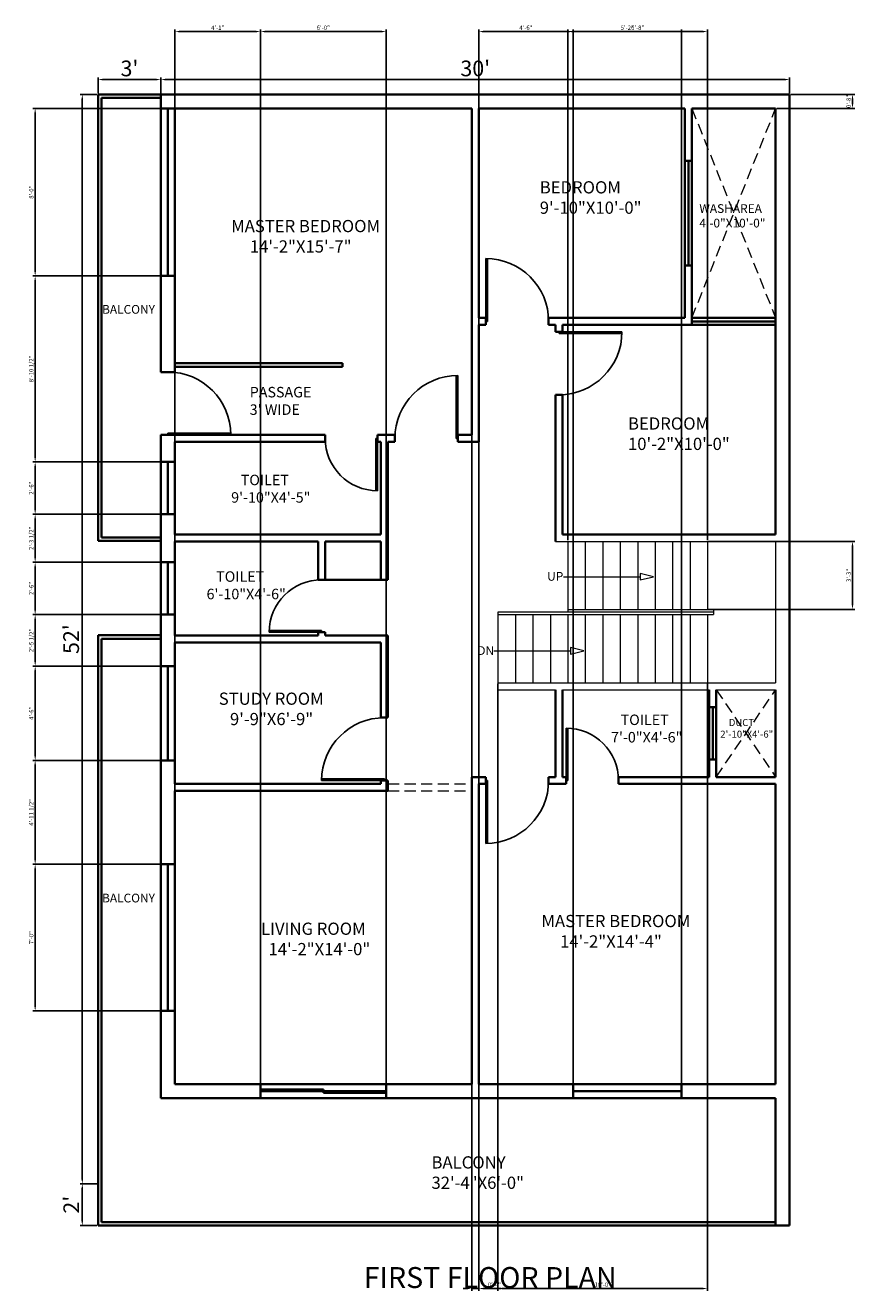
# Model space of a CAD drawing. Units: inches. Extents: x 1566 to 2546, y 1087 to 2705.
# Tile 27 of 27: x 2072 to 2546, y 1980 to 2705. Entities that reach past the tile are written whole.
import ezdxf

# ---------------------------------------------------------------- set-up
doc = ezdxf.new("R2010")
doc.units = ezdxf.units.IN
doc.linetypes.add('DASHED', pattern=[19.05, 12.7, -6.35])
for name, color, linetype, lineweight in [('A-ANNO-DIMS', 2, 'Continuous', 18), ('A-ANNO-TEXT', 7, 'Continuous', 18), ('A-AREA-IDEN', 7, 'Continuous', 18), ('A-DOOR', 4, 'Continuous', 25), ('A-FLOR-OVHD', 8, 'DASHED', 18), ('A-FLOR-STRS', 3, 'Continuous', 18), ('A-WALL', 7, 'Continuous', 35)]:
    doc.layers.add(name, color=color, linetype=linetype, lineweight=lineweight)
doc.styles.get("Standard").update_dxf_attribs({"font": 'arial.ttf'})
doc.dimstyles.new('ISO-25', dxfattribs={"dimtxt": 2.5, "dimasz": 2.5, "dimexe": 1.25, "dimexo": 0.625, "dimtad": 1, "dimtxsty": 'Standard', "dimcen": 2.5, "dimadec": 0, "dimazin": 0, "dimtfac": 1, "dimtmove": 0, "dimatfit": 3, "dimfxl": 1, "dimarcsym": 0})

# ---------------------------------------------------------------- blocks, each defined once
blk = doc.blocks.new('*D17')
at = {"layer": 'A-ANNO-DIMS', "color": 0, "lineweight": -2, "transparency": 16777216}
for p, q in [((2113.17, 2665.97), (2113.17, 2675.12)), ((2149.17, 2665.97), (2149.17, 2675.12)), ((2115.67, 2673.87), (2146.67, 2673.87))]:
    blk.add_line(p, q, dxfattribs=at)
at = {"layer": 'A-ANNO-DIMS', "color": 0, "transparency": 16777216}
for points in [[(2115.67, 2674.28), (2115.67, 2673.45), (2113.17, 2673.87)], [(2146.67, 2674.28), (2146.67, 2673.45), (2149.17, 2673.87)]]:
    blk.add_solid(points, dxfattribs=at)
at = {"layer": 'Defpoints', "color": 0, "transparency": 16777216}
for p in [(2149.17, 2673.87), (2113.17, 2665.35), (2149.17, 2665.35)]:
    blk.add_point(p, dxfattribs=at)
at = {"layer": 'A-ANNO-DIMS', "color": 0, "transparency": 16777216, "insert": (2131.17, 2679.09), "char_height": 9, "attachment_point": 5}
blk.add_mtext("3'", dxfattribs=at)
blk = doc.blocks.new('*D18')
at = {"layer": 'A-ANNO-DIMS', "color": 0, "lineweight": -2, "transparency": 16777216}
for p, q in [((2149.17, 2665.97), (2149.17, 2675.12)), ((2509.17, 2665.97), (2509.17, 2675.12)), ((2151.67, 2673.87), (2506.67, 2673.87))]:
    blk.add_line(p, q, dxfattribs=at)
at = {"layer": 'A-ANNO-DIMS', "color": 0, "transparency": 16777216}
for points in [[(2151.67, 2674.28), (2151.67, 2673.45), (2149.17, 2673.87)], [(2506.67, 2674.28), (2506.67, 2673.45), (2509.17, 2673.87)]]:
    blk.add_solid(points, dxfattribs=at)
at = {"layer": 'Defpoints', "color": 0, "transparency": 16777216}
for p in [(2509.17, 2673.87), (2149.17, 2665.35), (2509.17, 2665.35)]:
    blk.add_point(p, dxfattribs=at)
at = {"layer": 'A-ANNO-DIMS', "color": 0, "transparency": 16777216, "insert": (2329.17, 2679.09), "char_height": 9, "attachment_point": 5}
blk.add_mtext("30'", dxfattribs=at)
blk = doc.blocks.new('*D16')
at = {"layer": 'A-ANNO-DIMS', "color": 0, "lineweight": -2, "transparency": 16777216}
for p, q in [((2112.55, 2665.35), (2102.9, 2665.35)), ((2104.15, 2662.85), (2104.15, 2043.85)), ((2112.55, 2041.35), (2102.9, 2041.35))]:
    blk.add_line(p, q, dxfattribs=at)
at = {"layer": 'A-ANNO-DIMS', "color": 0, "transparency": 16777216}
for points in [[(2103.73, 2662.85), (2104.57, 2662.85), (2104.15, 2665.35)], [(2103.73, 2043.85), (2104.57, 2043.85), (2104.15, 2041.35)]]:
    blk.add_solid(points, dxfattribs=at)
at = {"layer": 'Defpoints', "color": 0, "transparency": 16777216}
for p in [(2113.17, 2665.35), (2104.15, 2041.35), (2113.17, 2041.35)]:
    blk.add_point(p, dxfattribs=at)
at = {"layer": 'A-ANNO-DIMS', "color": 0, "transparency": 16777216, "insert": (2098.93, 2353.35), "char_height": 9, "attachment_point": 5, "rotation": 90}
blk.add_mtext("52'", dxfattribs=at)
blk = doc.blocks.new('*D19')
at = {"layer": 'A-ANNO-DIMS', "color": 0, "lineweight": -2, "transparency": 16777216}
for p, q in [((2112.55, 2041.35), (2102.9, 2041.35)), ((2104.15, 2038.85), (2104.15, 2019.85)), ((2112.55, 2017.35), (2102.9, 2017.35))]:
    blk.add_line(p, q, dxfattribs=at)
at = {"layer": 'A-ANNO-DIMS', "color": 0, "transparency": 16777216}
for points in [[(2103.73, 2038.85), (2104.57, 2038.85), (2104.15, 2041.35)], [(2103.73, 2019.85), (2104.57, 2019.85), (2104.15, 2017.35)]]:
    blk.add_solid(points, dxfattribs=at)
at = {"layer": 'Defpoints', "color": 0, "transparency": 16777216}
for p in [(2113.17, 2041.35), (2104.15, 2017.35), (2113.17, 2017.35)]:
    blk.add_point(p, dxfattribs=at)
at = {"layer": 'A-ANNO-DIMS', "color": 0, "transparency": 16777216, "insert": (2099.01, 2029.35), "char_height": 9, "attachment_point": 5, "rotation": 90}
blk.add_mtext("2'", dxfattribs=at)
blk = doc.blocks.new('d1')
for p, q in [((3297.32, 1596.93), (3297.32, 1632.93)), ((3298.32, 1596.93), (3298.32, 1632.93)), ((3297.32, 1596.93), (3298.32, 1596.93))]:
    blk.add_line(p, q)
at = {"ltscale": 0.3}
blk.add_arc((3297.32, 1596.93), 36, 0, 90, dxfattribs=at)
blk = doc.blocks.new('d2')
for p, q in [((3364.08, 1632.29), (3364.08, 1602.29)), ((3365.08, 1632.29), (3365.08, 1602.29)), ((3364.08, 1602.29), (3365.08, 1602.29))]:
    blk.add_line(p, q)
at = {"ltscale": 0.3}
blk.add_arc((3364.08, 1602.29), 30, 0, 90, dxfattribs=at)
blk = doc.blocks.new('*D89')
at = {"layer": 'A-ANNO-DIMS', "color": 0, "lineweight": -2, "transparency": 16777216}
for p, q in [((2509.8, 2665.35), (2546.42, 2665.35)), ((2545.17, 2662.85), (2545.17, 2659.85)), ((2501.8, 2657.35), (2546.42, 2657.35))]:
    blk.add_line(p, q, dxfattribs=at)
at = {"layer": 'A-ANNO-DIMS', "color": 0, "transparency": 16777216}
for points in [[(2544.75, 2662.85), (2545.59, 2662.85), (2545.17, 2665.35)], [(2544.75, 2659.85), (2545.59, 2659.85), (2545.17, 2657.35)]]:
    blk.add_solid(points, dxfattribs=at)
at = {"layer": 'Defpoints', "color": 0, "transparency": 16777216}
for p in [(2509.17, 2665.35), (2501.17, 2657.35), (2545.17, 2657.35)]:
    blk.add_point(p, dxfattribs=at)
at = {"layer": 'A-ANNO-DIMS', "color": 0, "transparency": 16777216, "insert": (2543.27, 2661.35), "char_height": 2.5, "attachment_point": 5, "rotation": 90}
blk.add_mtext('0\'-8"', dxfattribs=at)
blk = doc.blocks.new('*D90')
at = {"layer": 'A-ANNO-DIMS', "color": 0, "lineweight": -2, "transparency": 16777216}
for p, q in [((2327.17, 2656.72), (2327.17, 1980.1)), ((2331.17, 2656.72), (2331.17, 1980.1)), ((2324.67, 1981.35), (2322.17, 1981.35)), ((2327.17, 1981.35), (2331.17, 1981.35)), ((2333.67, 1981.35), (2344.07, 1981.35))]:
    blk.add_line(p, q, dxfattribs=at)
at = {"layer": 'A-ANNO-DIMS', "color": 0, "transparency": 16777216}
for points in [[(2324.67, 1981.76), (2324.67, 1980.93), (2327.17, 1981.35)], [(2333.67, 1981.76), (2333.67, 1980.93), (2331.17, 1981.35)]]:
    blk.add_solid(points, dxfattribs=at)
at = {"layer": 'Defpoints', "color": 0, "transparency": 16777216}
for p in [(2327.17, 2657.35), (2331.17, 2657.35), (2331.17, 1981.35)]:
    blk.add_point(p, dxfattribs=at)
at = {"layer": 'A-ANNO-DIMS', "color": 0, "transparency": 16777216, "insert": (2340.12, 1983.25), "char_height": 2.5, "attachment_point": 5}
blk.add_mtext('0\'-4"', dxfattribs=at)
blk = doc.blocks.new('*D93')
at = {"layer": 'A-ANNO-DIMS', "color": 0, "lineweight": -2, "transparency": 16777216}
for p, q in [((2148.55, 2657.35), (2075.92, 2657.35)), ((2077.17, 2654.85), (2077.17, 2563.85)), ((2148.55, 2561.35), (2075.92, 2561.35))]:
    blk.add_line(p, q, dxfattribs=at)
at = {"layer": 'A-ANNO-DIMS', "color": 0, "transparency": 16777216}
for points in [[(2076.75, 2654.85), (2077.59, 2654.85), (2077.17, 2657.35)], [(2076.75, 2563.85), (2077.59, 2563.85), (2077.17, 2561.35)]]:
    blk.add_solid(points, dxfattribs=at)
at = {"layer": 'Defpoints', "color": 0, "transparency": 16777216}
for p in [(2149.17, 2657.35), (2077.17, 2561.35), (2149.17, 2561.35)]:
    blk.add_point(p, dxfattribs=at)
at = {"layer": 'A-ANNO-DIMS', "color": 0, "transparency": 16777216, "insert": (2075.27, 2609.35), "char_height": 2.5, "attachment_point": 5, "rotation": 90}
blk.add_mtext('8\'-0"', dxfattribs=at)
blk = doc.blocks.new('*D94')
at = {"layer": 'A-ANNO-DIMS', "color": 0, "lineweight": -2, "transparency": 16777216}
for p, q in [((2148.55, 2561.35), (2075.92, 2561.35)), ((2077.17, 2558.85), (2077.17, 2457.35)), ((2148.55, 2454.85), (2075.92, 2454.85))]:
    blk.add_line(p, q, dxfattribs=at)
at = {"layer": 'A-ANNO-DIMS', "color": 0, "transparency": 16777216}
for points in [[(2076.75, 2558.85), (2077.59, 2558.85), (2077.17, 2561.35)], [(2076.75, 2457.35), (2077.59, 2457.35), (2077.17, 2454.85)]]:
    blk.add_solid(points, dxfattribs=at)
at = {"layer": 'Defpoints', "color": 0, "transparency": 16777216}
for p in [(2149.17, 2561.35), (2077.17, 2454.85), (2149.17, 2454.85)]:
    blk.add_point(p, dxfattribs=at)
at = {"layer": 'A-ANNO-DIMS', "color": 0, "transparency": 16777216, "insert": (2075.25, 2508.1), "char_height": 2.5, "attachment_point": 5, "rotation": 90}
blk.add_mtext('8\'-10 1/2"', dxfattribs=at)
blk = doc.blocks.new('*D95')
at = {"layer": 'A-ANNO-DIMS', "color": 0, "lineweight": -2, "transparency": 16777216}
for p, q in [((2148.55, 2454.85), (2075.92, 2454.85)), ((2077.17, 2452.35), (2077.17, 2427.35)), ((2148.55, 2424.85), (2075.92, 2424.85))]:
    blk.add_line(p, q, dxfattribs=at)
at = {"layer": 'A-ANNO-DIMS', "color": 0, "transparency": 16777216}
for points in [[(2076.75, 2452.35), (2077.59, 2452.35), (2077.17, 2454.85)], [(2076.75, 2427.35), (2077.59, 2427.35), (2077.17, 2424.85)]]:
    blk.add_solid(points, dxfattribs=at)
at = {"layer": 'Defpoints', "color": 0, "transparency": 16777216}
for p in [(2149.17, 2454.85), (2077.17, 2424.85), (2149.17, 2424.85)]:
    blk.add_point(p, dxfattribs=at)
at = {"layer": 'A-ANNO-DIMS', "color": 0, "transparency": 16777216, "insert": (2075.27, 2439.85), "char_height": 2.5, "attachment_point": 5, "rotation": 90}
blk.add_mtext('2\'-6"', dxfattribs=at)
blk = doc.blocks.new('*D96')
at = {"layer": 'A-ANNO-DIMS', "color": 0, "lineweight": -2, "transparency": 16777216}
for p, q in [((2148.55, 2424.85), (2075.92, 2424.85)), ((2077.17, 2422.35), (2077.17, 2399.85)), ((2148.55, 2397.35), (2075.92, 2397.35))]:
    blk.add_line(p, q, dxfattribs=at)
at = {"layer": 'A-ANNO-DIMS', "color": 0, "transparency": 16777216}
for points in [[(2076.75, 2422.35), (2077.59, 2422.35), (2077.17, 2424.85)], [(2076.75, 2399.85), (2077.59, 2399.85), (2077.17, 2397.35)]]:
    blk.add_solid(points, dxfattribs=at)
at = {"layer": 'Defpoints', "color": 0, "transparency": 16777216}
for p in [(2149.17, 2424.85), (2077.17, 2397.35), (2149.17, 2397.35)]:
    blk.add_point(p, dxfattribs=at)
at = {"layer": 'A-ANNO-DIMS', "color": 0, "transparency": 16777216, "insert": (2075.25, 2411.1), "char_height": 2.5, "attachment_point": 5, "rotation": 90}
blk.add_mtext('2\'-3 1/2"', dxfattribs=at)
blk = doc.blocks.new('*D97')
at = {"layer": 'A-ANNO-DIMS', "color": 0, "lineweight": -2, "transparency": 16777216}
for p, q in [((2148.55, 2397.35), (2075.92, 2397.35)), ((2077.17, 2394.85), (2077.17, 2369.85)), ((2148.55, 2367.35), (2075.92, 2367.35))]:
    blk.add_line(p, q, dxfattribs=at)
at = {"layer": 'A-ANNO-DIMS', "color": 0, "transparency": 16777216}
for points in [[(2076.75, 2394.85), (2077.59, 2394.85), (2077.17, 2397.35)], [(2076.75, 2369.85), (2077.59, 2369.85), (2077.17, 2367.35)]]:
    blk.add_solid(points, dxfattribs=at)
at = {"layer": 'Defpoints', "color": 0, "transparency": 16777216}
for p in [(2149.17, 2397.35), (2077.17, 2367.35), (2149.17, 2367.35)]:
    blk.add_point(p, dxfattribs=at)
at = {"layer": 'A-ANNO-DIMS', "color": 0, "transparency": 16777216, "insert": (2075.27, 2382.35), "char_height": 2.5, "attachment_point": 5, "rotation": 90}
blk.add_mtext('2\'-6"', dxfattribs=at)
blk = doc.blocks.new('*D98')
at = {"layer": 'A-ANNO-DIMS', "color": 0, "lineweight": -2, "transparency": 16777216}
for p, q in [((2148.55, 2367.35), (2075.92, 2367.35)), ((2077.17, 2364.85), (2077.17, 2340.35)), ((2148.55, 2337.85), (2075.92, 2337.85))]:
    blk.add_line(p, q, dxfattribs=at)
at = {"layer": 'A-ANNO-DIMS', "color": 0, "transparency": 16777216}
for points in [[(2076.75, 2364.85), (2077.59, 2364.85), (2077.17, 2367.35)], [(2076.75, 2340.35), (2077.59, 2340.35), (2077.17, 2337.85)]]:
    blk.add_solid(points, dxfattribs=at)
at = {"layer": 'Defpoints', "color": 0, "transparency": 16777216}
for p in [(2149.17, 2367.35), (2077.17, 2337.85), (2149.17, 2337.85)]:
    blk.add_point(p, dxfattribs=at)
at = {"layer": 'A-ANNO-DIMS', "color": 0, "transparency": 16777216, "insert": (2075.25, 2352.6), "char_height": 2.5, "attachment_point": 5, "rotation": 90}
blk.add_mtext('2\'-5 1/2"', dxfattribs=at)
blk = doc.blocks.new('*D99')
at = {"layer": 'A-ANNO-DIMS', "color": 0, "lineweight": -2, "transparency": 16777216}
for p, q in [((2148.55, 2337.85), (2075.92, 2337.85)), ((2077.17, 2335.35), (2077.17, 2286.35)), ((2148.55, 2283.85), (2075.92, 2283.85))]:
    blk.add_line(p, q, dxfattribs=at)
at = {"layer": 'A-ANNO-DIMS', "color": 0, "transparency": 16777216}
for points in [[(2076.75, 2335.35), (2077.59, 2335.35), (2077.17, 2337.85)], [(2076.75, 2286.35), (2077.59, 2286.35), (2077.17, 2283.85)]]:
    blk.add_solid(points, dxfattribs=at)
at = {"layer": 'Defpoints', "color": 0, "transparency": 16777216}
for p in [(2149.17, 2337.85), (2077.17, 2283.85), (2149.17, 2283.85)]:
    blk.add_point(p, dxfattribs=at)
at = {"layer": 'A-ANNO-DIMS', "color": 0, "transparency": 16777216, "insert": (2075.27, 2310.85), "char_height": 2.5, "attachment_point": 5, "rotation": 90}
blk.add_mtext('4\'-6"', dxfattribs=at)
blk = doc.blocks.new('*D100')
at = {"layer": 'A-ANNO-DIMS', "color": 0, "lineweight": -2, "transparency": 16777216}
for p, q in [((2148.55, 2283.85), (2075.92, 2283.85)), ((2077.17, 2281.35), (2077.17, 2226.85)), ((2148.55, 2224.35), (2075.92, 2224.35))]:
    blk.add_line(p, q, dxfattribs=at)
at = {"layer": 'A-ANNO-DIMS', "color": 0, "transparency": 16777216}
for points in [[(2076.75, 2281.35), (2077.59, 2281.35), (2077.17, 2283.85)], [(2076.75, 2226.85), (2077.59, 2226.85), (2077.17, 2224.35)]]:
    blk.add_solid(points, dxfattribs=at)
at = {"layer": 'Defpoints', "color": 0, "transparency": 16777216}
for p in [(2149.17, 2283.85), (2077.17, 2224.35), (2149.17, 2224.35)]:
    blk.add_point(p, dxfattribs=at)
at = {"layer": 'A-ANNO-DIMS', "color": 0, "transparency": 16777216, "insert": (2075.25, 2254.1), "char_height": 2.5, "attachment_point": 5, "rotation": 90}
blk.add_mtext('4\'-11 1/2"', dxfattribs=at)
blk = doc.blocks.new('*D101')
at = {"layer": 'A-ANNO-DIMS', "color": 0, "lineweight": -2, "transparency": 16777216}
for p, q in [((2148.55, 2224.35), (2075.92, 2224.35)), ((2077.17, 2221.85), (2077.17, 2142.85)), ((2148.55, 2140.35), (2075.92, 2140.35))]:
    blk.add_line(p, q, dxfattribs=at)
at = {"layer": 'A-ANNO-DIMS', "color": 0, "transparency": 16777216}
for points in [[(2076.75, 2221.85), (2077.59, 2221.85), (2077.17, 2224.35)], [(2076.75, 2142.85), (2077.59, 2142.85), (2077.17, 2140.35)]]:
    blk.add_solid(points, dxfattribs=at)
at = {"layer": 'Defpoints', "color": 0, "transparency": 16777216}
for p in [(2149.17, 2224.35), (2077.17, 2140.35), (2149.17, 2140.35)]:
    blk.add_point(p, dxfattribs=at)
at = {"layer": 'A-ANNO-DIMS', "color": 0, "transparency": 16777216, "insert": (2075.27, 2182.35), "char_height": 2.5, "attachment_point": 5, "rotation": 90}
blk.add_mtext('7\'-0"', dxfattribs=at)
blk = doc.blocks.new('*D102')
at = {"layer": 'A-ANNO-DIMS', "color": 0, "lineweight": -2, "transparency": 16777216}
for p, q in [((2157.17, 2098.97), (2157.17, 2702.6)), ((2159.67, 2701.35), (2203.67, 2701.35)), ((2206.17, 2098.97), (2206.17, 2702.6))]:
    blk.add_line(p, q, dxfattribs=at)
at = {"layer": 'A-ANNO-DIMS', "color": 0, "transparency": 16777216}
for points in [[(2159.67, 2701.76), (2159.67, 2700.93), (2157.17, 2701.35)], [(2203.67, 2701.76), (2203.67, 2700.93), (2206.17, 2701.35)]]:
    blk.add_solid(points, dxfattribs=at)
at = {"layer": 'Defpoints', "color": 0, "transparency": 16777216}
for p in [(2206.17, 2701.35), (2157.17, 2098.35), (2206.17, 2098.35)]:
    blk.add_point(p, dxfattribs=at)
at = {"layer": 'A-ANNO-DIMS', "color": 0, "transparency": 16777216, "insert": (2181.67, 2703.23), "char_height": 2.5, "attachment_point": 5}
blk.add_mtext('4\'-1"', dxfattribs=at)
blk = doc.blocks.new('*D103')
at = {"layer": 'A-ANNO-DIMS', "color": 0, "lineweight": -2, "transparency": 16777216}
for p, q in [((2206.17, 2098.97), (2206.17, 2702.6)), ((2208.67, 2701.35), (2275.67, 2701.35)), ((2278.17, 2098.97), (2278.17, 2702.6))]:
    blk.add_line(p, q, dxfattribs=at)
at = {"layer": 'A-ANNO-DIMS', "color": 0, "transparency": 16777216}
for points in [[(2208.67, 2701.76), (2208.67, 2700.93), (2206.17, 2701.35)], [(2275.67, 2701.76), (2275.67, 2700.93), (2278.17, 2701.35)]]:
    blk.add_solid(points, dxfattribs=at)
at = {"layer": 'Defpoints', "color": 0, "transparency": 16777216}
for p in [(2278.17, 2701.35), (2206.17, 2098.35), (2278.17, 2098.35)]:
    blk.add_point(p, dxfattribs=at)
at = {"layer": 'A-ANNO-DIMS', "color": 0, "transparency": 16777216, "insert": (2242.17, 2703.25), "char_height": 2.5, "attachment_point": 5}
blk.add_mtext('6\'-0"', dxfattribs=at)
blk = doc.blocks.new('*D104')
at = {"layer": 'A-ANNO-DIMS', "color": 0, "lineweight": -2, "transparency": 16777216}
for p, q in [((2331.17, 2098.97), (2331.17, 2702.6)), ((2333.67, 2701.35), (2382.67, 2701.35)), ((2385.17, 2098.97), (2385.17, 2702.6))]:
    blk.add_line(p, q, dxfattribs=at)
at = {"layer": 'A-ANNO-DIMS', "color": 0, "transparency": 16777216}
for points in [[(2333.67, 2701.76), (2333.67, 2700.93), (2331.17, 2701.35)], [(2382.67, 2701.76), (2382.67, 2700.93), (2385.17, 2701.35)]]:
    blk.add_solid(points, dxfattribs=at)
at = {"layer": 'Defpoints', "color": 0, "transparency": 16777216}
for p in [(2385.17, 2701.35), (2331.17, 2098.35), (2385.17, 2098.35)]:
    blk.add_point(p, dxfattribs=at)
at = {"layer": 'A-ANNO-DIMS', "color": 0, "transparency": 16777216, "insert": (2358.17, 2703.25), "char_height": 2.5, "attachment_point": 5}
blk.add_mtext('4\'-6"', dxfattribs=at)
blk = doc.blocks.new('*D105')
at = {"layer": 'A-ANNO-DIMS', "color": 0, "lineweight": -2, "transparency": 16777216}
for p, q in [((2385.17, 2098.97), (2385.17, 2702.6)), ((2387.67, 2701.35), (2444.67, 2701.35)), ((2447.17, 2098.97), (2447.17, 2702.6))]:
    blk.add_line(p, q, dxfattribs=at)
at = {"layer": 'A-ANNO-DIMS', "color": 0, "transparency": 16777216}
for points in [[(2387.67, 2701.76), (2387.67, 2700.93), (2385.17, 2701.35)], [(2444.67, 2701.76), (2444.67, 2700.93), (2447.17, 2701.35)]]:
    blk.add_solid(points, dxfattribs=at)
at = {"layer": 'Defpoints', "color": 0, "transparency": 16777216}
for p in [(2447.17, 2701.35), (2385.17, 2098.35), (2447.17, 2098.35)]:
    blk.add_point(p, dxfattribs=at)
at = {"layer": 'A-ANNO-DIMS', "color": 0, "transparency": 16777216, "insert": (2416.17, 2703.25), "char_height": 2.5, "attachment_point": 5}
blk.add_mtext('5\'-2"', dxfattribs=at)
blk = doc.blocks.new('*D106')
at = {"layer": 'A-ANNO-DIMS', "color": 0, "lineweight": -2, "transparency": 16777216}
for p, q in [((2382.17, 2409.97), (2382.17, 2702.6)), ((2384.67, 2701.35), (2459.67, 2701.35)), ((2462.17, 2409.97), (2462.17, 2702.6))]:
    blk.add_line(p, q, dxfattribs=at)
at = {"layer": 'A-ANNO-DIMS', "color": 0, "transparency": 16777216}
for points in [[(2384.67, 2701.76), (2384.67, 2700.93), (2382.17, 2701.35)], [(2459.67, 2701.76), (2459.67, 2700.93), (2462.17, 2701.35)]]:
    blk.add_solid(points, dxfattribs=at)
at = {"layer": 'Defpoints', "color": 0, "transparency": 16777216}
for p in [(2462.17, 2701.35), (2382.17, 2409.35), (2462.17, 2409.35)]:
    blk.add_point(p, dxfattribs=at)
at = {"layer": 'A-ANNO-DIMS', "color": 0, "transparency": 16777216, "insert": (2422.17, 2703.25), "char_height": 2.5, "attachment_point": 5}
blk.add_mtext('6\'-8"', dxfattribs=at)
blk = doc.blocks.new('*D107')
at = {"layer": 'A-ANNO-DIMS', "color": 0, "lineweight": -2, "transparency": 16777216}
for p, q in [((2462.8, 2409.35), (2546.42, 2409.35)), ((2545.17, 2406.85), (2545.17, 2372.85)), ((2462.8, 2370.35), (2546.42, 2370.35))]:
    blk.add_line(p, q, dxfattribs=at)
at = {"layer": 'A-ANNO-DIMS', "color": 0, "transparency": 16777216}
for points in [[(2544.75, 2406.85), (2545.59, 2406.85), (2545.17, 2409.35)], [(2544.75, 2372.85), (2545.59, 2372.85), (2545.17, 2370.35)]]:
    blk.add_solid(points, dxfattribs=at)
at = {"layer": 'Defpoints', "color": 0, "transparency": 16777216}
for p in [(2462.17, 2409.35), (2462.17, 2370.35), (2545.17, 2370.35)]:
    blk.add_point(p, dxfattribs=at)
at = {"layer": 'A-ANNO-DIMS', "color": 0, "transparency": 16777216, "insert": (2543.27, 2389.85), "char_height": 2.5, "attachment_point": 5, "rotation": 90}
blk.add_mtext('3\'-3"', dxfattribs=at)
blk = doc.blocks.new('*D108')
at = {"layer": 'A-ANNO-DIMS', "color": 0, "lineweight": -2, "transparency": 16777216}
for p, q in [((2342.17, 2327.72), (2342.17, 1980.1)), ((2462.17, 2327.72), (2462.17, 1980.1)), ((2344.67, 1981.35), (2459.67, 1981.35))]:
    blk.add_line(p, q, dxfattribs=at)
at = {"layer": 'A-ANNO-DIMS', "color": 0, "transparency": 16777216}
for points in [[(2344.67, 1981.76), (2344.67, 1980.93), (2342.17, 1981.35)], [(2459.67, 1981.76), (2459.67, 1980.93), (2462.17, 1981.35)]]:
    blk.add_solid(points, dxfattribs=at)
at = {"layer": 'Defpoints', "color": 0, "transparency": 16777216}
for p in [(2342.17, 2328.35), (2462.17, 2328.35), (2462.17, 1981.35)]:
    blk.add_point(p, dxfattribs=at)
at = {"layer": 'A-ANNO-DIMS', "color": 0, "transparency": 16777216, "insert": (2402.17, 1983.25), "char_height": 2.5, "attachment_point": 5}
blk.add_mtext('10\'-0"', dxfattribs=at)

msp = doc.modelspace()

# ---------------------------------------------------------------- linework, layer by layer
at = {"layer": 'A-FLOR-OVHD', "ltscale": 0.5}
for p, q in [((2453.17, 2657.35), (2501.17, 2537.35)), ((2453.17, 2537.35), (2501.17, 2657.35)), ((2467.17, 2324.35), (2501.17, 2274.35)), ((2467.17, 2274.35), (2501.17, 2324.35)), ((2279.17, 2270.35), (2327.17, 2270.35)), ((2279.17, 2266.35), (2327.17, 2266.35))]:
    msp.add_line(p, q, dxfattribs=at)
at = {"layer": 'A-FLOR-STRS'}
for p, q in [((2375.17, 2409.35), (2501.17, 2409.35)), ((2382.17, 2409.35), (2382.17, 2368.85)), ((2392.17, 2409.35), (2392.17, 2370.35)), ((2402.17, 2409.35), (2402.17, 2370.35)), ((2412.17, 2409.35), (2412.17, 2370.35)), ((2422.17, 2409.35), (2422.17, 2370.35)), ((2432.17, 2409.35), (2432.17, 2370.35)), ((2442.17, 2409.35), (2442.17, 2370.35)), ((2452.17, 2409.35), (2452.17, 2370.35)), ((2462.17, 2409.35), (2462.17, 2370.35)), ((2501.17, 2409.35), (2501.17, 2328.35)), ((2379.74, 2389.1), (2423.62, 2389.1)), ((2382.17, 2370.35), (2465.67, 2370.35)), ((2465.67, 2370.35), (2465.67, 2367.35)), ((2342.17, 2368.85), (2342.17, 2324.35)), ((2465.67, 2368.85), (2342.17, 2368.85)), ((2342.17, 2367.35), (2465.67, 2367.35)), ((2352.17, 2367.35), (2352.17, 2328.35)), ((2362.17, 2367.35), (2362.17, 2328.35)), ((2372.17, 2367.35), (2372.17, 2328.35)), ((2382.17, 2367.35), (2382.17, 2366.85)), ((2382.17, 2367.35), (2382.17, 2328.35)), ((2392.17, 2367.35), (2392.17, 2328.35)), ((2402.17, 2367.35), (2402.17, 2328.35)), ((2412.17, 2367.35), (2412.17, 2328.35)), ((2422.17, 2367.35), (2422.17, 2328.35)), ((2432.17, 2367.35), (2432.17, 2328.35)), ((2442.17, 2367.35), (2442.17, 2328.35)), ((2452.17, 2367.35), (2452.17, 2328.35)), ((2462.17, 2367.35), (2462.17, 2328.35)), ((2339.74, 2346.6), (2383.62, 2346.6)), ((2342.17, 2328.35), (2501.17, 2328.35)), ((2342.17, 2324.35), (2375.17, 2324.35)), ((2379.17, 2324.35), (2463.17, 2324.35)), ((2467.17, 2324.35), (2501.17, 2324.35))]:
    msp.add_line(p, q, dxfattribs=at)
for points in [[(2431.27, 2389.1), (2423.62, 2390.95), (2423.62, 2387.24)], [(2391.27, 2346.6), (2383.62, 2348.45), (2383.62, 2344.74)]]:
    msp.add_lwpolyline(points, close=True, dxfattribs=at)
at = {"layer": 'A-WALL'}
for p, q in [((2113.17, 2409.59), (2113.17, 2665.35)), ((2113.17, 2665.35), (2149.17, 2665.35)), ((2115.17, 2411.59), (2115.17, 2663.35)), ((2115.17, 2663.35), (2149.17, 2663.35)), ((2149.17, 2506.35), (2149.17, 2665.35)), ((2149.17, 2665.35), (2509.17, 2665.35)), ((2509.17, 2665.35), (2509.17, 2017.35)), ((2149.17, 2657.35), (2327.17, 2657.35)), ((2153.17, 2561.35), (2153.17, 2657.35)), ((2157.17, 2506.35), (2157.17, 2657.35)), ((2327.17, 2470.35), (2327.17, 2657.35)), ((2331.17, 2657.35), (2449.17, 2657.35)), ((2331.17, 2537.35), (2331.17, 2657.35)), ((2449.17, 2537.35), (2449.17, 2657.35)), ((2453.17, 2657.35), (2501.17, 2657.35)), ((2453.17, 2533.35), (2453.17, 2657.35)), ((2501.17, 2657.35), (2501.17, 2413.35)), ((2449.17, 2627.35), (2453.17, 2627.35)), ((2451.17, 2627.35), (2451.17, 2567.35)), ((2449.17, 2567.35), (2453.17, 2567.35)), ((2149.17, 2561.35), (2157.17, 2561.35)), ((2331.17, 2537.35), (2335.17, 2537.35)), ((2335.17, 2533.35), (2335.17, 2537.35)), ((2371.17, 2537.35), (2449.17, 2537.35)), ((2371.17, 2533.35), (2371.17, 2537.35)), ((2453.17, 2537.35), (2501.17, 2537.35)), ((2331.17, 2533.35), (2335.17, 2533.35)), ((2331.17, 2466.35), (2331.17, 2533.35)), ((2371.17, 2533.35), (2375.17, 2533.35)), ((2375.17, 2533.35), (2375.17, 2529.35)), ((2379.17, 2533.35), (2501.17, 2533.35)), ((2379.17, 2533.35), (2379.17, 2529.35)), ((2501.17, 2535.35), (2453.17, 2535.35)), ((2375.17, 2529.35), (2379.17, 2529.35)), ((2157.17, 2511.35), (2253.17, 2511.35)), ((2157.17, 2509.35), (2253.17, 2509.35)), ((2253.17, 2509.35), (2253.17, 2511.35)), ((2149.17, 2506.35), (2157.17, 2506.35)), ((2375.17, 2493.35), (2379.17, 2493.35)), ((2375.17, 2493.35), (2375.17, 2409.35)), ((2379.17, 2493.35), (2379.17, 2413.35)), ((2149.17, 2090.35), (2149.17, 2470.35)), ((2149.17, 2470.35), (2243.17, 2470.35)), ((2157.17, 2466.35), (2243.17, 2466.35)), ((2157.17, 2413.35), (2157.17, 2466.35)), ((2243.17, 2466.35), (2243.17, 2470.35)), ((2273.17, 2470.35), (2275.17, 2470.35)), ((2273.17, 2466.35), (2273.17, 2470.35)), ((2273.17, 2466.35), (2275.17, 2466.35)), ((2275.17, 2470.35), (2283.17, 2470.35)), ((2275.17, 2413.35), (2275.17, 2466.35)), ((2279.17, 2466.35), (2283.17, 2466.35)), ((2279.17, 2387.35), (2279.17, 2466.35)), ((2283.17, 2466.35), (2283.17, 2470.35)), ((2319.17, 2470.35), (2327.17, 2470.35)), ((2319.17, 2466.35), (2319.17, 2470.35)), ((2319.17, 2466.35), (2331.17, 2466.35)), ((2157.17, 2454.85), (2149.17, 2454.85)), ((2153.17, 2454.85), (2153.17, 2424.85)), ((2157.17, 2424.85), (2149.17, 2424.85)), ((2149.17, 2409.59), (2113.17, 2409.59)), ((2149.17, 2411.59), (2115.17, 2411.59)), ((2157.17, 2413.35), (2275.17, 2413.35)), ((2157.17, 2409.35), (2239.17, 2409.35)), ((2157.17, 2355.35), (2157.17, 2409.35)), ((2239.17, 2387.35), (2239.17, 2409.35)), ((2243.17, 2409.35), (2275.17, 2409.35)), ((2243.17, 2387.35), (2243.17, 2409.35)), ((2275.17, 2387.35), (2275.17, 2409.35)), ((2379.17, 2413.35), (2501.17, 2413.35)), ((2157.17, 2397.35), (2149.17, 2397.35)), ((2153.17, 2397.35), (2153.17, 2367.35)), ((2239.17, 2387.35), (2279.17, 2387.35)), ((2157.17, 2367.35), (2149.17, 2367.35)), ((2239.17, 2355.35), (2239.17, 2357.35)), ((2239.17, 2357.35), (2243.17, 2357.35)), ((2243.17, 2355.35), (2243.17, 2357.35)), ((2149.17, 2355.56), (2113.17, 2355.56)), ((2113.17, 2355.56), (2113.17, 2017.35)), ((2149.17, 2353.56), (2115.17, 2353.56)), ((2115.17, 2353.56), (2115.17, 2019.35)), ((2157.17, 2355.35), (2239.17, 2355.35)), ((2157.17, 2351.35), (2275.17, 2351.35)), ((2157.17, 2270.35), (2157.17, 2351.35)), ((2243.17, 2355.35), (2279.17, 2355.35)), ((2275.17, 2308.35), (2275.17, 2351.35)), ((2279.17, 2308.35), (2279.17, 2355.35)), ((2157.17, 2337.85), (2149.17, 2337.85)), ((2153.17, 2337.85), (2153.17, 2283.85)), ((2375.17, 2324.35), (2375.17, 2274.35)), ((2379.17, 2324.35), (2379.17, 2274.35)), ((2463.17, 2324.35), (2463.17, 2274.35)), ((2467.17, 2324.35), (2467.17, 2274.35)), ((2501.17, 2324.35), (2501.17, 2274.35)), ((2463.17, 2314.35), (2467.17, 2314.35)), ((2465.17, 2314.35), (2465.17, 2284.35)), ((2275.17, 2308.35), (2279.17, 2308.35)), ((2157.17, 2283.85), (2149.17, 2283.85)), ((2463.17, 2284.35), (2467.17, 2284.35)), ((2157.17, 2270.35), (2275.17, 2270.35)), ((2275.17, 2272.35), (2279.17, 2272.35)), ((2275.17, 2270.35), (2275.17, 2272.35)), ((2279.17, 2266.35), (2279.17, 2272.35)), ((2327.17, 2274.35), (2335.17, 2274.35)), ((2327.17, 2098.35), (2327.17, 2274.35)), ((2331.17, 2270.35), (2335.17, 2270.35)), ((2331.17, 2098.35), (2331.17, 2270.35)), ((2335.17, 2270.35), (2335.17, 2274.35)), ((2371.17, 2274.35), (2375.17, 2274.35)), ((2371.17, 2270.35), (2371.17, 2274.35)), ((2371.17, 2270.35), (2381.17, 2270.35)), ((2379.17, 2274.35), (2381.17, 2274.35)), ((2381.17, 2274.35), (2381.17, 2270.35)), ((2411.17, 2274.35), (2463.17, 2274.35)), ((2411.17, 2274.35), (2411.17, 2270.35)), ((2411.17, 2270.35), (2501.17, 2270.35)), ((2467.17, 2274.35), (2501.17, 2274.35)), ((2501.17, 2270.35), (2501.17, 2098.35)), ((2157.17, 2266.35), (2279.17, 2266.35)), ((2157.17, 2098.35), (2157.17, 2266.35)), ((2157.17, 2224.35), (2149.17, 2224.35)), ((2153.17, 2224.35), (2153.17, 2140.35)), ((2157.17, 2140.35), (2149.17, 2140.35)), ((2157.17, 2098.35), (2327.17, 2098.35)), ((2206.17, 2098.35), (2206.17, 2090.35)), ((2206.17, 2095.35), (2242.17, 2095.35)), ((2242.17, 2095.35), (2242.17, 2093.35)), ((2278.17, 2098.35), (2278.17, 2090.35)), ((2331.17, 2098.35), (2501.17, 2098.35)), ((2385.17, 2098.35), (2385.17, 2090.35)), ((2447.17, 2098.35), (2447.17, 2090.35)), ((2149.17, 2090.35), (2501.17, 2090.35)), ((2206.17, 2094.35), (2278.17, 2094.35)), ((2242.17, 2093.35), (2278.17, 2093.35)), ((2385.17, 2094.35), (2447.17, 2094.35)), ((2501.17, 2090.35), (2501.17, 2017.35)), ((2113.17, 2017.35), (2509.17, 2017.35)), ((2115.17, 2019.35), (2501.17, 2019.35))]:
    msp.add_line(p, q, dxfattribs=at)

# ---------------------------------------------------------------- block references
at = {"layer": 'A-DOOR'}
for name, p in [('d1', (-962.15, 938.42)), ('d2', (-982.91, 670.05))]:
    msp.add_blockref(name, p, dxfattribs=at)
for name, p, rotation in [('d1', (780.25, 5826.67), 270), ('d2', (5637.25, 4070.64), 180), ('d2', (3843.46, -1006.73), 90), ('d1', (3874.1, -1024.98), 90)]:
    msp.add_blockref(name, p, dxfattribs=dict(at, rotation=rotation))
at = {"layer": 'A-DOOR', "xscale": -1}
for p, rotation in [((556.25, -826.98), 270), ((-962.15, 3869.27), 180)]:
    msp.add_blockref('d1', p, dxfattribs=dict(at, rotation=rotation))
msp.add_blockref('d1', (5616.49, 871.42), dxfattribs=at)

# ---------------------------------------------------------------- texts
at = {"layer": 'A-ANNO-TEXT'}
for s, p in [('UP', (2370.32, 2386.79)), ('DN', (2330.32, 2344.29))]:
    msp.add_text(s, height=5, dxfattribs=at).set_placement(p)
at = {"layer": 'A-AREA-IDEN', "attachment_point": 1}
for s, width, insert, char_height in [('BEDROOM\\P9\'-10"X10\'-0"', 111.7553, (2366.1, 2615.64), 7), ('WASHAREA\\P4\'-0"X10\'-0"', 111.7553, (2457.49, 2602.49), 5), ('MASTER BEDROOM\\P     14\'-2"X15\'-7"', 111.7553, (2189.39, 2593.45), 7), ('BALCONY', 111.7553, (2115.46, 2544.74), 5), ("PASSAGE\\P3' WIDE", 111.7553, (2200.02, 2497.81), 6), ('BEDROOM\\P10\'-2"X10\'-0"', 111.7553, (2416.62, 2480.35), 7), ('   TOILET\\P9\'-10"X4\'-5"', 111.7553, (2189.39, 2447.51), 6), ('   TOILET\\P6\'-10"X4\'-6"', 111.7553, (2175.3, 2392.18), 6), ('STUDY ROOM\\P   9\'-9"X6\'-9"', 111.7553, (2182.29, 2322.72), 7), ('   TOILET\\P7\'-0"X4\'-6"', 111.7553, (2406.89, 2310.13), 6), ('    DUCT\\P2\'-10"X4\'-6"', 111.7553, (2469.47, 2307.57), 4), ('BALCONY', 111.7553, (2115.46, 2207.52), 5), ('LIVING ROOM\\P  14\'-2"X14\'-0"', 111.7553, (2206.51, 2190.94), 7), ('MASTER BEDROOM\\P     14\'-2"X14\'-4"', 111.7553, (2367.05, 2195.34), 7), ('BALCONY\\P32\'-4"X6\'-0"', 111.7553, (2304.11, 2057.09), 7), ('FIRST FLOOR PLAN', 179.2212, (2265.35, 1993.63), 12)]:
    msp.add_mtext_dynamic_manual_height_columns(s, width=width, gutter_width=12.5, heights=[0], dxfattribs=dict(at, insert=insert, char_height=char_height))

# ---------------------------------------------------------------- dimensions: what is measured, and where the dimension line sits
at = {"layer": 'A-ANNO-DIMS'}
for base, p1, p2, override, picture, middle in [((2206.17, 2701.35), (2157.17, 2098.35), (2206.17, 2098.35), {"dimdec": 1, "dimlfac": 1, "dimrnd": 0, "dimzin": 1, "dimdsep": 46, "dimlunit": 4, "dimfrac": 2}, '*D102', (2181.67, 2703.23)), ((2278.17, 2701.35), (2206.17, 2098.35), (2278.17, 2098.35), {"dimdec": 1, "dimlfac": 1, "dimrnd": 0, "dimzin": 1, "dimdsep": 46, "dimlunit": 4, "dimfrac": 2}, '*D103', (2242.17, 2703.25)), ((2385.17, 2701.35), (2331.17, 2098.35), (2385.17, 2098.35), {"dimdec": 1, "dimlfac": 1, "dimrnd": 0, "dimzin": 1, "dimdsep": 46, "dimlunit": 4, "dimfrac": 2}, '*D104', (2358.17, 2703.25)), ((2462.17, 2701.35), (2382.17, 2409.35), (2462.17, 2409.35), {"dimdec": 1, "dimlfac": 1, "dimrnd": 0, "dimzin": 1, "dimdsep": 46, "dimlunit": 4, "dimfrac": 2}, '*D106', (2422.17, 2703.25)), ((2447.17, 2701.35), (2385.17, 2098.35), (2447.17, 2098.35), {"dimdec": 1, "dimlfac": 1, "dimrnd": 0, "dimzin": 1, "dimdsep": 46, "dimlunit": 4, "dimfrac": 2}, '*D105', (2416.17, 2703.25)), ((2149.17, 2673.87), (2113.17, 2665.35), (2149.17, 2665.35), {"dimtxt": 9, "dimdec": 1, "dimlunit": 3, "dimclrd": 0, "dimclre": 0, "dimclrt": 0, "dimtdec": 1}, '*D17', (2131.17, 2679.09)), ((2509.17, 2673.87), (2149.17, 2665.35), (2509.17, 2665.35), {"dimtxt": 9, "dimdec": 1, "dimlunit": 3, "dimclrd": 0, "dimclre": 0, "dimclrt": 0, "dimtdec": 1, "dimtmove": 1}, '*D18', (2329.17, 2679.09)), ((2331.17, 1981.35), (2327.17, 2657.35), (2331.17, 2657.35), {"dimdec": 1, "dimlfac": 1, "dimrnd": 0, "dimzin": 1, "dimdsep": 46, "dimlunit": 4, "dimfrac": 2}, '*D90', (2340.12, 1983.25)), ((2462.17, 1981.35), (2342.17, 2328.35), (2462.17, 2328.35), {"dimdec": 1, "dimlfac": 1, "dimrnd": 0, "dimzin": 1, "dimdsep": 46, "dimlunit": 4, "dimfrac": 2}, '*D108', (2402.17, 1983.25))]:
    dim = msp.add_linear_dim(base=base, p1=p1, p2=p2, dimstyle='ISO-25', override=override, dxfattribs=at)
    dim.commit()
    dim.dimension.update_dxf_attribs({"geometry": picture, "text_midpoint": middle})
for base, p1, p2, override, picture, middle in [((2104.15, 2041.35), (2113.17, 2665.35), (2113.17, 2041.35), {"dimtxt": 9, "dimdec": 1, "dimlunit": 3, "dimclrd": 0, "dimclre": 0, "dimclrt": 0, "dimtdec": 1}, '*D16', (2098.93, 2353.35)), ((2545.17, 2657.35), (2509.17, 2665.35), (2501.17, 2657.35), {"dimdec": 1, "dimlfac": 1, "dimrnd": 0, "dimzin": 1, "dimdsep": 46, "dimlunit": 4, "dimfrac": 2}, '*D89', (2543.27, 2661.35)), ((2077.17, 2561.35), (2149.17, 2657.35), (2149.17, 2561.35), {"dimdec": 1, "dimlfac": 1, "dimrnd": 0, "dimzin": 1, "dimdsep": 46, "dimlunit": 4, "dimfrac": 2}, '*D93', (2075.27, 2609.35)), ((2077.17, 2454.85), (2149.17, 2561.35), (2149.17, 2454.85), {"dimdec": 1, "dimlfac": 1, "dimrnd": 0, "dimzin": 1, "dimdsep": 46, "dimlunit": 4, "dimfrac": 2}, '*D94', (2075.25, 2508.1)), ((2077.17, 2424.85), (2149.17, 2454.85), (2149.17, 2424.85), {"dimdec": 1, "dimlfac": 1, "dimrnd": 0, "dimzin": 1, "dimdsep": 46, "dimlunit": 4, "dimfrac": 2}, '*D95', (2075.27, 2439.85)), ((2077.17, 2397.35), (2149.17, 2424.85), (2149.17, 2397.35), {"dimdec": 1, "dimlfac": 1, "dimrnd": 0, "dimzin": 1, "dimdsep": 46, "dimlunit": 4, "dimfrac": 2}, '*D96', (2075.25, 2411.1)), ((2545.17, 2370.35), (2462.17, 2409.35), (2462.17, 2370.35), {"dimdec": 1, "dimlfac": 1, "dimrnd": 0, "dimzin": 1, "dimdsep": 46, "dimlunit": 4, "dimfrac": 2}, '*D107', (2543.27, 2389.85)), ((2077.17, 2367.35), (2149.17, 2397.35), (2149.17, 2367.35), {"dimdec": 1, "dimlfac": 1, "dimrnd": 0, "dimzin": 1, "dimdsep": 46, "dimlunit": 4, "dimfrac": 2}, '*D97', (2075.27, 2382.35)), ((2077.17, 2337.85), (2149.17, 2367.35), (2149.17, 2337.85), {"dimdec": 1, "dimlfac": 1, "dimrnd": 0, "dimzin": 1, "dimdsep": 46, "dimlunit": 4, "dimfrac": 2}, '*D98', (2075.25, 2352.6)), ((2077.17, 2283.85), (2149.17, 2337.85), (2149.17, 2283.85), {"dimdec": 1, "dimlfac": 1, "dimrnd": 0, "dimzin": 1, "dimdsep": 46, "dimlunit": 4, "dimfrac": 2}, '*D99', (2075.27, 2310.85)), ((2077.17, 2224.35), (2149.17, 2283.85), (2149.17, 2224.35), {"dimdec": 1, "dimlfac": 1, "dimrnd": 0, "dimzin": 1, "dimdsep": 46, "dimlunit": 4, "dimfrac": 2}, '*D100', (2075.25, 2254.1)), ((2077.17, 2140.35), (2149.17, 2224.35), (2149.17, 2140.35), {"dimdec": 1, "dimlfac": 1, "dimrnd": 0, "dimzin": 1, "dimdsep": 46, "dimlunit": 4, "dimfrac": 2}, '*D101', (2075.27, 2182.35)), ((2104.15, 2017.35), (2113.17, 2041.35), (2113.17, 2017.35), {"dimtxt": 9, "dimdec": 1, "dimlunit": 3, "dimclrd": 0, "dimclre": 0, "dimclrt": 0, "dimtdec": 1, "dimtmove": 1}, '*D19', (2099.01, 2029.35))]:
    dim = msp.add_linear_dim(base=base, p1=p1, p2=p2, angle=90, dimstyle='ISO-25', override=override, dxfattribs=at)
    dim.commit()
    dim.dimension.update_dxf_attribs({"geometry": picture, "text_midpoint": middle})

doc.saveas('drawing.dxf')
